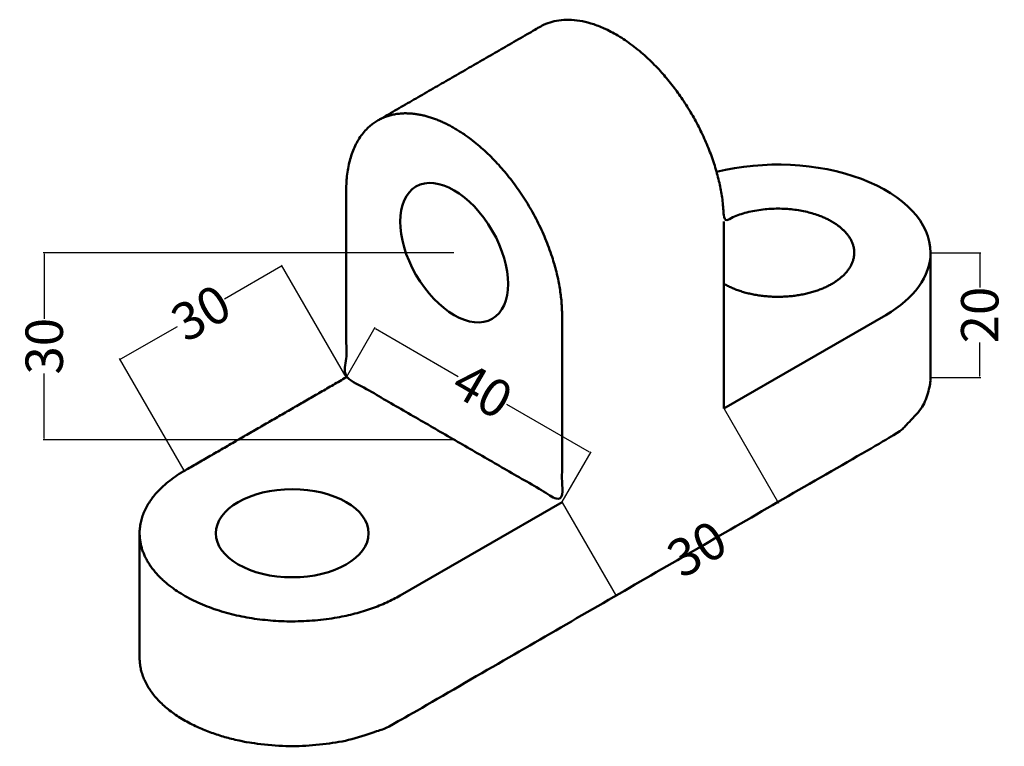
# Model space of a CAD drawing. Units: millimetres. Extents: x -7 to 151, y 27 to 144.
import ezdxf

# ---------------------------------------------------------------- set-up
doc = ezdxf.new("R2010")
doc.units = ezdxf.units.MM
doc.header["$MEASUREMENT"] = 0
doc.layers.add('M-DIMS', color=2, linetype='Continuous', lineweight=25)
doc.layers.add('M-OUTL', color=7, linetype='Continuous', lineweight=50)
doc.styles.get("Standard").update_dxf_attribs({"font": 'arial.ttf'})
doc.dimstyles.get("Standard").update_dxf_attribs({"dimtxt": 6, "dimasz": 0.18, "dimexe": 0.18, "dimexo": 0.0625, "dimgap": 0.09, "dimtad": 0, "dimtoh": 1, "dimdec": 0, "dimzin": 0, "dimdsep": 46, "dimtxsty": 'Standard', "dimcen": 0.09, "dimadec": 0, "dimazin": 0, "dimtfac": 1, "dimtdec": 0, "dimtofl": 0, "dimtmove": 0, "dimatfit": 3, "dimfxl": 1, "dimtolj": 1, "dimtzin": 0, "dimarcsym": 0})

# ---------------------------------------------------------------- blocks, each defined once
blk = doc.blocks.new('*D1')
at = {"layer": 'Defpoints', "color": 0, "transparency": 16777216}
for p in [(106.13, 81.52), (80.15, 66.52), (114.79, 66.52)]:
    blk.add_point(p, dxfattribs=at)
at = {"layer": 'M-DIMS', "color": 0, "lineweight": -2, "transparency": 16777216}
for p, q in [((106.16, 81.47), (114.88, 66.36)), ((80.18, 66.47), (88.9, 51.36)), ((114.64, 66.43), (105.59, 61.21)), ((88.97, 51.61), (98.01, 56.83))]:
    blk.add_line(p, q, dxfattribs=at)
at = {"layer": 'M-DIMS', "color": 0, "transparency": 16777216}
for points in [[(114.62, 66.46), (114.65, 66.4), (114.79, 66.52)], [(88.95, 51.64), (88.98, 51.58), (88.81, 51.52)]]:
    blk.add_solid(points, dxfattribs=at)
at = {"layer": 'M-DIMS', "color": 0, "transparency": 16777216, "insert": (101.8, 59.02), "char_height": 6, "attachment_point": 5, "rotation": 30}
blk.add_mtext('\\A1;30', dxfattribs=at)
blk = doc.blocks.new('*D2')
at = {"layer": 'Defpoints', "color": 0, "transparency": 16777216}
for p in [(45.51, 86.52), (84.72, 74.43), (80.15, 66.52)]:
    blk.add_point(p, dxfattribs=at)
at = {"layer": 'M-DIMS', "color": 0, "lineweight": -2, "transparency": 16777216}
for p, q in [((45.54, 86.57), (50.17, 94.59)), ((50.23, 94.34), (63.5, 86.68)), ((84.56, 74.52), (71.29, 82.18)), ((80.18, 66.57), (84.81, 74.59))]:
    blk.add_line(p, q, dxfattribs=at)
at = {"layer": 'M-DIMS', "color": 0, "transparency": 16777216}
for points in [[(50.25, 94.37), (50.22, 94.31), (50.08, 94.43)], [(84.58, 74.55), (84.55, 74.49), (84.72, 74.43)]]:
    blk.add_solid(points, dxfattribs=at)
at = {"layer": 'M-DIMS', "color": 0, "transparency": 16777216, "insert": (67.4, 84.43), "char_height": 6, "attachment_point": 5, "rotation": 330}
blk.add_mtext('\\A1;40', dxfattribs=at)
blk = doc.blocks.new('*D3')
at = {"layer": 'Defpoints', "color": 0, "transparency": 16777216}
for p in [(35.2, 104.38), (45.51, 86.52), (19.53, 71.52)]:
    blk.add_point(p, dxfattribs=at)
at = {"layer": 'M-DIMS', "color": 0, "lineweight": -2, "transparency": 16777216}
for p, q in [((35.04, 104.29), (26, 99.07)), ((45.48, 86.57), (35.11, 104.54)), ((9.37, 89.47), (18.42, 94.69)), ((19.5, 71.57), (9.13, 89.54))]:
    blk.add_line(p, q, dxfattribs=at)
at = {"layer": 'M-DIMS', "color": 0, "transparency": 16777216}
for points in [[(35.03, 104.32), (35.06, 104.27), (35.2, 104.38)], [(9.36, 89.5), (9.39, 89.45), (9.22, 89.38)]]:
    blk.add_solid(points, dxfattribs=at)
at = {"layer": 'M-DIMS', "color": 0, "transparency": 16777216, "insert": (22.21, 96.88), "char_height": 6, "attachment_point": 5, "rotation": 30}
blk.add_mtext('\\A1;30', dxfattribs=at)
blk = doc.blocks.new('*D4')
at = {"layer": 'Defpoints', "color": 0, "transparency": 16777216}
for p in [(139.29, 106.52), (139.29, 86.52), (147.18, 86.52)]:
    blk.add_point(p, dxfattribs=at)
at = {"layer": 'M-DIMS', "color": 0, "lineweight": -2, "transparency": 16777216}
for p, q in [((139.35, 106.52), (147.36, 106.52)), ((147.18, 106.34), (147.18, 100.95)), ((147.18, 86.7), (147.18, 92.09)), ((139.35, 86.52), (147.36, 86.52))]:
    blk.add_line(p, q, dxfattribs=at)
at = {"layer": 'M-DIMS', "color": 0, "transparency": 16777216}
for points in [[(147.15, 106.34), (147.21, 106.34), (147.18, 106.52)], [(147.15, 86.7), (147.21, 86.7), (147.18, 86.52)]]:
    blk.add_solid(points, dxfattribs=at)
at = {"layer": 'M-DIMS', "color": 0, "transparency": 16777216, "insert": (147.18, 96.52), "char_height": 6, "attachment_point": 5, "rotation": 90}
blk.add_mtext('\\A1;20', dxfattribs=at)
blk = doc.blocks.new('*D5')
at = {"layer": 'Defpoints', "color": 0, "transparency": 16777216}
for p in [(62.83, 106.52), (-2.95, 76.52), (62.83, 76.52)]:
    blk.add_point(p, dxfattribs=at)
at = {"layer": 'M-DIMS', "color": 0, "lineweight": -2, "transparency": 16777216}
for p, q in [((62.77, 106.52), (-3.13, 106.52)), ((-2.95, 106.34), (-2.95, 95.9)), ((-2.95, 76.7), (-2.95, 87.14)), ((62.77, 76.52), (-3.13, 76.52))]:
    blk.add_line(p, q, dxfattribs=at)
at = {"layer": 'M-DIMS', "color": 0, "transparency": 16777216}
for points in [[(-2.98, 106.34), (-2.92, 106.34), (-2.95, 106.52)], [(-2.98, 76.7), (-2.92, 76.7), (-2.95, 76.52)]]:
    blk.add_solid(points, dxfattribs=at)
at = {"layer": 'M-DIMS', "color": 0, "transparency": 16777216, "insert": (-2.95, 91.52), "char_height": 6, "attachment_point": 5, "rotation": 90}
blk.add_mtext('\\A1;30', dxfattribs=at)

msp = doc.modelspace()

# ---------------------------------------------------------------- linework, layer by layer
at = {"layer": 'M-OUTL'}
for p, q in [((106.13, 81.52), (106.13, 111.52)), ((106.13, 81.52), (132.11, 96.52)), ((54.17, 51.52), (80.15, 66.52))]:
    msp.add_line(p, q, dxfattribs=at)
for start_param, end_param in [(0, 1.98436), (5.497787, 6.283185)]:
    msp.add_ellipse((114.79, 106.52), major_axis=(24.49, 0), ratio=0.57735, start_param=start_param, end_param=end_param, dxfattribs=at)
for centre, major_axis in [((62.83, 106.52), (6.12, -10.61)), ((36.85, 61.52), (-12.25, 0))]:
    msp.add_ellipse(centre, major_axis=major_axis, ratio=0.57735, dxfattribs=at)
for points, weights, knots in [([(106.13, 101.52), (114.79, 96.52), (123.45, 101.52), (132.11, 106.52), (123.45, 111.52), (114.79, 116.52), (106.13, 111.52), (106.13, 124.88), (95.44, 136.17), (84.75, 147.46), (76.57, 142.73), (63.57, 135.23), (50.58, 127.73)], [1, 0.707106781187, 1, 0.707106781187, 1, 0.707106781187, 1, 0.831469612303, 1, 0.831469612303, 1, 1, 1], [0, 0, 0, 1.570796, 1.570796, 3.141593, 3.141593, 4.712389, 4.712389, 5.890486, 5.890486, 7.068583, 7.068583, 8.068583, 8.068583, 8.068583]), ([(80.15, 96.52), (80.15, 108.07), (71.49, 118.84), (62.83, 129.61), (54.17, 128.84), (45.51, 128.07), (45.51, 116.52), (45.51, 101.52), (45.51, 86.52), (62.83, 76.52), (80.15, 66.52), (80.15, 81.52), (80.15, 96.52)], [1, 0.866025403784, 1, 0.866025403784, 1, 0.866025403784, 1, 1, 1, 1, 1, 1, 1], [0, 0, 0, 1.047198, 1.047198, 2.094395, 2.094395, 3.141593, 3.141593, 4.141593, 4.141593, 5.141593, 5.141593, 6.141593, 6.141593, 6.141593]), ([(12.36, 61.52), (12.36, 51.52), (12.36, 41.52), (12.36, 32.07), (27.48, 28.45), (42.6, 24.84), (54.17, 31.52), (93.14, 54.02), (132.11, 76.52), (139.29, 80.66), (139.29, 86.52), (139.29, 96.52), (139.29, 106.52)], [1, 1, 1, 0.831469612303, 1, 0.831469612303, 1, 1, 1, 0.923879532511, 1, 1, 1], [0, 0, 0, 1, 1, 2.178097, 2.178097, 3.356194, 3.356194, 4.356194, 4.356194, 5.141593, 5.141593, 6.141593, 6.141593, 6.141593]), ([(45.51, 86.52), (32.52, 79.02), (19.53, 71.52), (9.53, 65.75), (13.19, 57.86), (16.85, 49.97), (30.51, 47.86), (44.17, 45.75), (54.17, 51.52)], [1, 1, 1, 0.866025403784, 1, 0.866025403784, 1, 0.866025403784, 1], [0, 0, 0, 1, 1, 2.047198, 2.047198, 3.094395, 3.094395, 4.141593, 4.141593, 4.141593])]:
    msp.add_rational_spline(points, weights, degree=2, knots=knots, dxfattribs=at)

# ---------------------------------------------------------------- dimensions: what is measured, and where the dimension line sits
at = {"layer": 'M-DIMS'}
for p1, p2, distance, picture, middle in [((62.83, 106.52), (62.83, 76.52), -65.78, '*D5', (-2.95, 91.52)), ((139.29, 106.52), (139.29, 86.52), 7.89, '*D4', (147.18, 96.52)), ((19.53, 71.52), (45.51, 86.52), 20.62, '*D3', (22.21, 96.88)), ((45.51, 86.52), (80.15, 66.52), 9.13, '*D2', (67.4, 84.43)), ((80.15, 66.52), (106.13, 81.52), -17.32, '*D1', (101.8, 59.02))]:
    dim = msp.add_aligned_dim(p1=p1, p2=p2, distance=distance, dimstyle='Standard', override={"dimclrd": 0, "dimclre": 0, "dimclrt": 0}, dxfattribs=at)
    dim.commit()
    dim.dimension.update_dxf_attribs({"geometry": picture, "text_midpoint": middle})

doc.saveas('drawing.dxf')
